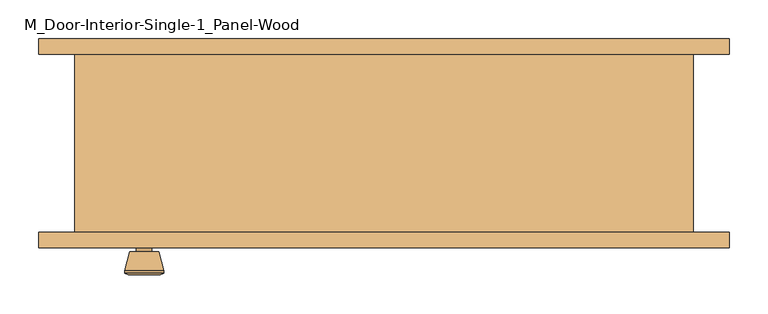
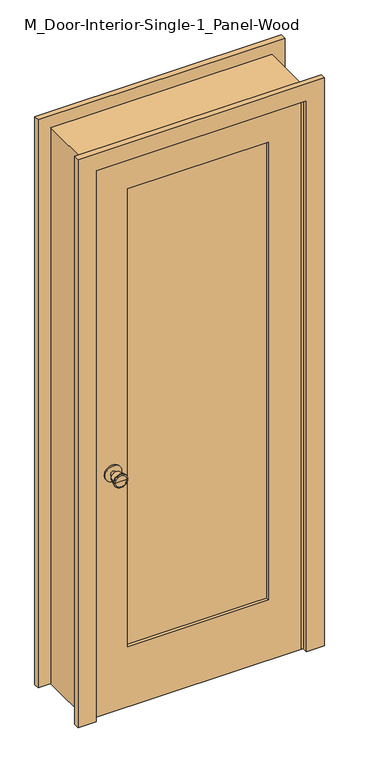
"""IFC4 building model written with IfcOpenShell, lengths in millimetres: door geometry, M_Door-Interior-Single-1_Panel-Wood."""

from ifc_helpers import new_model, si_unit, point, frame, frame_2d, origin, place, context, project, spatial, polyline, circle_curve, trimmed, segment, composite_curve, outline, extrude, faceted_brep, source, transform, mapped, element, save
from ifc_brep_helpers import plane_surface, cylinder_surface, revolved_surface, advanced_brep


def m_door_interior_single_1_panel_wood_1ba8bb0f(model_context):
    return source(origin(), model_context, "Body", "SolidModel", [
        advanced_brep(
        [(-310.0, -70.825, 914.4), (-320.0, -70.825, 914.4), (-300.0, -70.825, 914.4), (-289.5241324, -21.825, 914.4), (-330.4758676, -21.825, 914.4), (-310.0, -21.825, 914.4), (-285.0, -23.6528681, 914.4), (-335.0, -23.6528681, 914.4), (-285.0, -27.1165463, 914.4), (-335.0, -27.1165463, 914.4), (-291.363764, -51.825, 914.4), (-328.636236, -51.825, 914.4), (-300.0, -51.825, 914.4), (-320.0, -51.825, 914.4)],
        [
            (0, 1),
            (1, 2, circle_curve(frame((-310.0, -70.825, 914.4), z_axis=(0.0, -1.0, 0.0), x_axis=(-1.0, 0.0, 0.0)), 10.0)),
            (2, 0),
            (2, 1, circle_curve(frame((-310.0, -70.825, 914.4), z_axis=(0.0, -1.0, 0.0), x_axis=(-1.0, 0.0, 0.0)), 10.0)),
            (3, 4, circle_curve(frame((-310.0, -21.825, 914.4), z_axis=(0.0, 1.0, 0.0), x_axis=(-1.0, 0.0, 0.0)), 20.4758676)),
            (4, 5),
            (5, 3),
            (4, 3, circle_curve(frame((-310.0, -21.825, 914.4), z_axis=(0.0, 1.0, 0.0), x_axis=(-1.0, 0.0, 0.0)), 20.4758676)),
            (6, 7, circle_curve(frame((-310.0, -23.6528681, 914.4), z_axis=(0.0, 1.0, 0.0), x_axis=(-1.0, 0.0, 0.0)), 25.0)),
            (7, 4),
            (3, 6),
            (7, 6, circle_curve(frame((-310.0, -23.6528681, 914.4), z_axis=(0.0, 1.0, 0.0), x_axis=(-1.0, 0.0, 0.0)), 25.0)),
            (8, 9, circle_curve(frame((-310.0, -27.1165463, 914.4), z_axis=(0.0, 1.0, 0.0), x_axis=(-1.0, 0.0, 0.0)), 25.0)),
            (9, 7),
            (6, 8),
            (9, 8, circle_curve(frame((-310.0, -27.1165463, 914.4), z_axis=(0.0, 1.0, 0.0), x_axis=(-1.0, 0.0, 0.0)), 25.0)),
            (10, 11, circle_curve(frame((-310.0, -51.825, 914.4), z_axis=(0.0, 1.0, 0.0), x_axis=(-1.0, 0.0, 0.0)), 18.636236)),
            (11, 9),
            (8, 10),
            (11, 10, circle_curve(frame((-310.0, -51.825, 914.4), z_axis=(0.0, 1.0, 0.0), x_axis=(-1.0, 0.0, 0.0)), 18.636236)),
            (12, 13, circle_curve(frame((-310.0, -51.825, 914.4), z_axis=(0.0, 1.0, 0.0), x_axis=(-1.0, 0.0, 0.0)), 10.0)),
            (13, 11),
            (10, 12),
            (13, 12, circle_curve(frame((-310.0, -51.825, 914.4), z_axis=(0.0, 1.0, 0.0), x_axis=(-1.0, 0.0, 0.0)), 10.0)),
            (1, 13),
            (12, 2),
        ],
        [
            plane_surface(frame((-310.0, -70.825, 914.4), z_axis=(0.0, -1.0, 0.0), x_axis=(-1.0, 0.0, 0.0))),
            plane_surface(frame((-310.0, -21.825, 914.4), z_axis=(0.0, 1.0, 0.0), x_axis=(-1.0, 0.0, 0.0))),
            revolved_surface(polyline([(-330.4758676, -21.825, 914.4), (-335.0, -23.6528681, 914.4)]), (-310.0, -70.825, 914.4), (0.0, -1.0, 0.0)),
            cylinder_surface(frame((-310.0, -70.825, 914.4), z_axis=(0.0, -1.0, 0.0), x_axis=(-1.0, 0.0, 0.0)), 25.0),
            revolved_surface(polyline([(-335.0, -27.1165463, 914.4), (-328.636236, -51.825, 914.4)]), (-310.0, -70.825, 914.4), (0.0, -1.0, 0.0)),
            plane_surface(frame((-310.0, -51.825, 914.4), z_axis=(0.0, -1.0, 0.0), x_axis=(-1.0, 0.0, 0.0))),
            cylinder_surface(frame((-310.0, -70.825, 914.4), z_axis=(0.0, -1.0, 0.0), x_axis=(-1.0, 0.0, 0.0)), 10.0),
        ],
        [
            (0, [[1, 2, 3]]),
            (0, [[-3, 4, -1]]),
            (1, [[5, 6, 7]]),
            (1, [[8, -7, -6]]),
            (2, [[9, 10, -5, 11]]),
            (2, [[12, -11, -8, -10]]),
            (3, [[13, 14, -9, 15]]),
            (3, [[16, -15, -12, -14]]),
            (4, [[17, 18, -13, 19]]),
            (4, [[20, -19, -16, -18]]),
            (5, [[21, 22, -17, 23]]),
            (5, [[24, -23, -20, -22]]),
            (6, [[-2, 25, -21, 26]]),
            (6, [[-4, -26, -24, -25]]),
        ],
    ),
        extrude(outline(composite_curve([segment(trimmed(circle_curve(frame_2d((914.4, -310.0)), 30.0), [point((914.4, -340.0))], [point((914.4, -280.0))], False, "CARTESIAN"), True, "CONTINUOUS"), segment(trimmed(circle_curve(frame_2d((914.4, -310.0)), 30.0), [point((914.4, -280.0))], [point((914.4, -340.0))], False, "CARTESIAN"), True, "CONTINUOUS")], self_intersect=False)), frame((0.0, -76.825, 0.0), z_axis=(0.0, 1.0, 0.0), x_axis=(0.0, 0.0, 1.0)), (0.0, 0.0, 1.0), 6.0),
        advanced_brep(
        [(-310.0, -117.825, 914.4), (-300.0, -117.825, 914.4), (-320.0, -117.825, 914.4), (-289.5241324, -166.825, 914.4), (-310.0, -166.825, 914.4), (-330.4758676, -166.825, 914.4), (-285.0, -164.9971319, 914.4), (-335.0, -164.9971319, 914.4), (-285.0, -161.5334537, 914.4), (-335.0, -161.5334537, 914.4), (-291.363764, -136.825, 914.4), (-328.636236, -136.825, 914.4), (-300.0, -136.825, 914.4), (-320.0, -136.825, 914.4)],
        [
            (0, 1),
            (1, 2, circle_curve(frame((-310.0, -117.825, 914.4), z_axis=(0.0, 1.0, 0.0), x_axis=(-1.0, 0.0, 0.0)), 10.0)),
            (2, 0),
            (2, 1, circle_curve(frame((-310.0, -117.825, 914.4), z_axis=(0.0, 1.0, 0.0), x_axis=(-1.0, 0.0, 0.0)), 10.0)),
            (3, 4),
            (4, 5),
            (5, 3, circle_curve(frame((-310.0, -166.825, 914.4), z_axis=(0.0, -1.0, 0.0), x_axis=(-1.0, 0.0, 0.0)), 20.4758676)),
            (3, 5, circle_curve(frame((-310.0, -166.825, 914.4), z_axis=(0.0, -1.0, 0.0), x_axis=(-1.0, 0.0, 0.0)), 20.4758676)),
            (6, 3),
            (5, 7),
            (7, 6, circle_curve(frame((-310.0, -164.9971319, 914.4), z_axis=(0.0, -1.0, 0.0), x_axis=(-1.0, 0.0, 0.0)), 25.0)),
            (6, 7, circle_curve(frame((-310.0, -164.9971319, 914.4), z_axis=(0.0, -1.0, 0.0), x_axis=(-1.0, 0.0, 0.0)), 25.0)),
            (8, 6),
            (7, 9),
            (9, 8, circle_curve(frame((-310.0, -161.5334537, 914.4), z_axis=(0.0, -1.0, 0.0), x_axis=(-1.0, 0.0, 0.0)), 25.0)),
            (8, 9, circle_curve(frame((-310.0, -161.5334537, 914.4), z_axis=(0.0, -1.0, 0.0), x_axis=(-1.0, 0.0, 0.0)), 25.0)),
            (10, 8),
            (9, 11),
            (11, 10, circle_curve(frame((-310.0, -136.825, 914.4), z_axis=(0.0, -1.0, 0.0), x_axis=(-1.0, 0.0, 0.0)), 18.636236)),
            (10, 11, circle_curve(frame((-310.0, -136.825, 914.4), z_axis=(0.0, -1.0, 0.0), x_axis=(-1.0, 0.0, 0.0)), 18.636236)),
            (12, 10),
            (11, 13),
            (13, 12, circle_curve(frame((-310.0, -136.825, 914.4), z_axis=(0.0, -1.0, 0.0), x_axis=(-1.0, 0.0, 0.0)), 10.0)),
            (12, 13, circle_curve(frame((-310.0, -136.825, 914.4), z_axis=(0.0, -1.0, 0.0), x_axis=(-1.0, 0.0, 0.0)), 10.0)),
            (1, 12),
            (13, 2),
        ],
        [
            plane_surface(frame((-310.0, -117.825, 914.4), z_axis=(0.0, 1.0, 0.0), x_axis=(-1.0, 0.0, 0.0))),
            plane_surface(frame((-310.0, -166.825, 914.4), z_axis=(0.0, -1.0, 0.0), x_axis=(-1.0, 0.0, 0.0))),
            revolved_surface(polyline([(-330.4758676, -166.825, 914.4), (-335.0, -164.9971319, 914.4)]), (-310.0, -117.825, 914.4), (0.0, 1.0, 0.0)),
            cylinder_surface(frame((-310.0, -117.825, 914.4), z_axis=(0.0, 1.0, 0.0), x_axis=(-1.0, 0.0, 0.0)), 25.0),
            revolved_surface(polyline([(-335.0, -161.5334537, 914.4), (-328.636236, -136.825, 914.4)]), (-310.0, -117.825, 914.4), (0.0, 1.0, 0.0)),
            plane_surface(frame((-310.0, -136.825, 914.4), z_axis=(0.0, 1.0, 0.0), x_axis=(-1.0, 0.0, 0.0))),
            cylinder_surface(frame((-310.0, -117.825, 914.4), z_axis=(0.0, 1.0, 0.0), x_axis=(-1.0, 0.0, 0.0)), 10.0),
        ],
        [
            (0, [[1, 2, 3]]),
            (0, [[-3, 4, -1]]),
            (1, [[5, 6, 7]]),
            (1, [[-6, -5, 8]]),
            (2, [[9, -7, 10, 11]]),
            (2, [[-10, -8, -9, 12]]),
            (3, [[13, -11, 14, 15]]),
            (3, [[-14, -12, -13, 16]]),
            (4, [[17, -15, 18, 19]]),
            (4, [[-18, -16, -17, 20]]),
            (5, [[21, -19, 22, 23]]),
            (5, [[-22, -20, -21, 24]]),
            (6, [[25, -23, 26, -2]]),
            (6, [[-26, -24, -25, -4]]),
        ],
    ),
        extrude(outline(composite_curve([segment(trimmed(circle_curve(frame_2d((914.4, -310.0)), 30.0), [point((914.4, -340.0))], [point((914.4, -280.0))], False, "CARTESIAN"), True, "CONTINUOUS"), segment(trimmed(circle_curve(frame_2d((914.4, -310.0)), 30.0), [point((914.4, -280.0))], [point((914.4, -340.0))], False, "CARTESIAN"), True, "CONTINUOUS")], self_intersect=False)), frame((0.0, -117.825, 0.0), z_axis=(0.0, 1.0, 0.0), x_axis=(0.0, 0.0, 1.0)), (0.0, 0.0, 1.0), 6.0),
        faceted_brep([(400.0, -111.825, 0.0), (375.0, -111.825, 0.0), (375.0, -76.825, 0.0), (362.3, -76.825, 0.0), (362.3, -41.9, 0.0), (375.0, -41.9, 0.0), (375.0, 118.175, 0.0), (400.0, 118.175, 0.0), (400.0, 118.175, 2125.0), (400.0, -111.825, 2125.0), (375.0, 118.175, 2100.0), (-375.0, 118.175, 2100.0), (-375.0, 118.175, 0.0), (-400.0, 118.175, 0.0), (-400.0, 118.175, 2125.0), (375.0, -41.9, 2100.0), (362.3, -41.9, 2087.3), (-362.3, -41.9, 2087.3), (-362.3, -41.9, 0.0), (-375.0, -41.9, 0.0), (-375.0, -41.9, 2100.0), (362.3, -76.825, 2087.3), (375.0, -76.825, 2100.0), (-375.0, -76.825, 2100.0), (-375.0, -76.825, 0.0), (-362.3, -76.825, 0.0), (-362.3, -76.825, 2087.3), (375.0, -111.825, 2100.0), (-400.0, -111.825, 2125.0), (-400.0, -111.825, 0.0), (-375.0, -111.825, 0.0), (-375.0, -111.825, 2100.0)], [[[0, 1, 2, 3, 4, 5, 6, 7]], [[7, 8, 9, 0]], [[6, 10, 11, 12, 13, 14, 8, 7]], [[5, 15, 10, 6]], [[4, 16, 17, 18, 19, 20, 15, 5]], [[3, 21, 16, 4]], [[2, 22, 23, 24, 25, 26, 21, 3]], [[1, 27, 22, 2]], [[0, 9, 28, 29, 30, 31, 27, 1]], [[8, 14, 28, 9]], [[15, 20, 11, 10]], [[21, 26, 17, 16]], [[27, 31, 23, 22]], [[29, 13, 12, 19, 18, 25, 24, 30]], [[14, 13, 29, 28]], [[20, 19, 12, 11]], [[26, 25, 18, 17]], [[31, 30, 24, 23]]]),
        extrude(outline(polyline([(2100.0, -375.0), (0.0, -375.0), (0.0, 375.0), (2100.0, 375.0), (2100.0, -375.0)]), holes=[polyline([(1980.0, -255.0), (1980.0, 255.0), (230.0, 255.0), (230.0, -255.0), (1980.0, -255.0)])]), frame((0.0, -111.825, 0.0), z_axis=(0.0, 1.0, 0.0), x_axis=(0.0, 0.0, 1.0)), (0.0, 0.0, 1.0), 35.0),
        extrude(outline(polyline([(255.0, -88.4916667), (255.0, -100.1583333), (-255.0, -100.1583333), (-255.0, -88.4916667), (255.0, -88.4916667)])), frame((0.0, 0.0, 230.0), z_axis=(0.0, 0.0, 1.0), x_axis=(1.0, 0.0, 0.0)), (0.0, 0.0, 1.0), 1750.0),
        extrude(outline(polyline([(0.0, 446.35), (2171.35, 446.35), (2171.35, -446.35), (0.0, -446.35), (0.0, -381.35), (2106.35, -381.35), (2106.35, 381.35), (0.0, 381.35), (0.0, 446.35)])), frame((0.0, -131.825, 0.0), z_axis=(0.0, 1.0, 0.0), x_axis=(0.0, 0.0, 1.0)), (0.0, 0.0, 1.0), 20.0),
        extrude(outline(polyline([(0.0, 446.35), (2171.35, 446.35), (2171.35, -446.35), (0.0, -446.35), (0.0, -381.35), (2106.35, -381.35), (2106.35, 381.35), (0.0, 381.35), (0.0, 446.35)])), frame((0.0, 118.175, 0.0), z_axis=(0.0, 1.0, 0.0), x_axis=(0.0, 0.0, 1.0)), (0.0, 0.0, 1.0), 20.0),
    ])


if __name__ == "__main__":
    model = new_model("IFC4")
    model_context = context("Model", 3, world=origin())
    ifc_project = project(units=[si_unit("LENGTHUNIT", "METRE", prefix="MILLI")], contexts=[model_context])
    site = spatial("IfcSite", under=ifc_project)
    building = spatial("IfcBuilding", under=site)
    placement = place(None, origin())
    m_door_interior_single_1_panel_wood_shape = m_door_interior_single_1_panel_wood_1ba8bb0f(model_context)
    element("IfcDoor", 1, ObjectType="M_Door-Interior-Single-1_Panel-Wood", at=placement, inside=building, context=model_context, shape_type="MappedRepresentation", body=[
        mapped(m_door_interior_single_1_panel_wood_shape, transform((0.0, 0.0, 0.0), x_axis=(1.0, 0.0, 0.0), y_axis=(0.0, 1.0, 0.0), z_axis=(0.0, 0.0, 1.0))),
    ])
    save(model, "model.ifc")

# Revit data of these elements
# Type "M_Door-Interior-Single-1_Panel-Wood"
#   Type Mark = "23"
#   Assembly Code = "C1020300"
#   Analytic Construction = "Wooden"
#   Top Rail = 120 mm
#   Thickness = 35 mm
#   Thermal Resistance (R) = 0.455703 (m²·K)/W
#   Swing Angle [instance default] = 90.00°
#   Stiles = 120 mm
#   Rough Width = 800 mm
#   Rough Height = 2125 mm
#   Height = 2100 mm
#   Width = 750 mm
#   Heat Transfer Coefficient (U) = 2.19465 W/(m²·K)
#   Bottom Rail = 230 mm
#   Trim Material = Cherry
#   Panel Material = Cherry
#   Frame Material = Cherry
#   Door Handle Material = Aluminum
#   Visual Light Transmittance = 0
#   Solar Heat Gain Coefficient = 0
#   Wall Closure = (empty or 0)
#   Function = (empty or 0)
# Element 1 (IfcDoor, "M_Door-Interior-Single-1_Panel-Wood")
#   Materials on its faces: "Cherry", "Aluminum"
# Materials
#   "Cherry": class "Wood", colour RGB 154 107 61, transparency 0, Description = "Prunus Serotina", Cost = 0
#   "Aluminum": class "Metal", colour RGB 244 244 244, transparency 0, Description = "Aluminum 6061", Cost = 0
